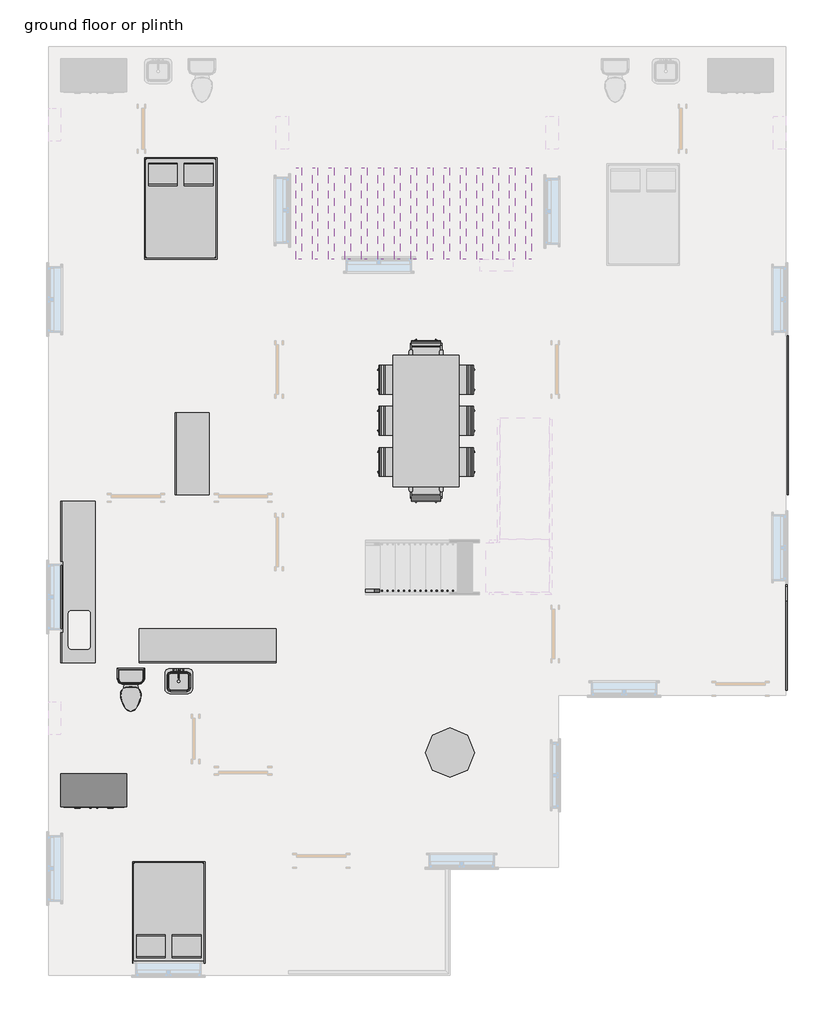
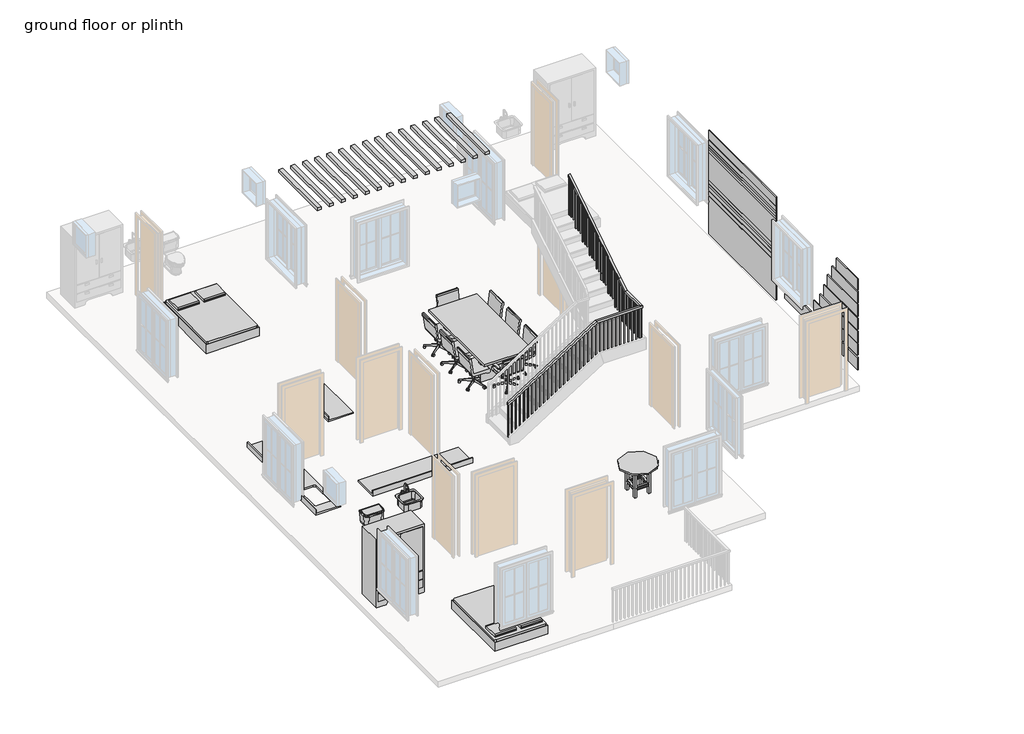
# One storey, part 2 of 3: 33 furniture elements, 2 flow terminals, 1 railing.
"""IFC4 building model written with IfcOpenShell, lengths in millimetres."""

from ifc_helpers import new_model, si_unit, frame, origin, place, context, project, spatial, polyline, outline, extrude, faceted_brep, transform, mapped, element, save
from components import flow_terminal_8d9ea526, toilet_domestic_3d_toilet_domestic_3d_ba6479b0, toilet_domestic_3d_toilet_domestic_3d_30431060, furniture_b58f7881, casework_1_casework_1_f574b021, casework_10_casework_1_3750556f, casework_11_casework_1_2f257332, casework_12_casework_1_dcbad799, casework_13_casework_1_b548bcc5, casework_14_casework_1_ad7f4f76, casework_16_casework_16_0ac3b185, casework_17_casework_17_3fc012a0, casework_18_casework_1_4256c183, casework_2_casework_1_1fe19027, casework_3_casework_1_f196c302, casework_4_casework_1_a5b175c9, casework_5_casework_1_a4356d40, casework_6_casework_1_aba422e7, casework_7_casework_1_d1433357, casework_8_casework_1_82254010, casework_9_casework_1_7a666160, chair_task_chair_task_b7f3823b, chair_task_arms_chair_task_arms_fa5a08ef, furniture_c0b19bce, furniture_c0b61535, furniture_6f689152, furniture_ec754799, furniture_32cec9f0, furniture_82e269c4

model = new_model("IFC4")

# Units and contexts
model_context = context("Model", 3, world=origin())
ifc_project = project(units=[si_unit("LENGTHUNIT", "METRE", prefix="MILLI")], contexts=[model_context])

# Site, building, storey
site = spatial("IfcSite", under=ifc_project)
building = spatial("IfcBuilding", under=site)
storey = spatial("IfcBuildingStorey", under=building, Name="ground floor or plinth", Elevation=609.6)

# Flow terminals
placement = place(None, origin())
flow_terminal_shape = flow_terminal_8d9ea526(model_context)
element("IfcFlowTerminal", 1, ObjectType="Sink Vanity-Square : 20\" x 18\"", at=placement, inside=storey, context=model_context, shape_type="MappedRepresentation", body=[
    mapped(flow_terminal_shape, transform((3106.5030862, 5324.1042913, 609.6), x_axis=(1.0, 0.0, 0.0), y_axis=(0.0, 1.0, 0.0), z_axis=(0.0, 0.0, 1.0))),
])
toilet_domestic_3d_toilet_domestic_3d_shape = toilet_domestic_3d_toilet_domestic_3d_ba6479b0(model_context)
toilet_domestic_3d_toilet_domestic_3d_2_shape = toilet_domestic_3d_toilet_domestic_3d_30431060(model_context)
element("IfcFlowTerminal", 2, ObjectType="Toilet-Domestic-3D : Toilet-Domestic-3D", at=placement, inside=storey, context=model_context, shape_type="MappedRepresentation", body=[
    mapped(toilet_domestic_3d_toilet_domestic_3d_shape, transform((2233.1923267, 5021.6496924, 609.6), x_axis=(1.0, 0.0, 0.0), y_axis=(0.0, 1.0, 0.0), z_axis=(0.0, 0.0, 1.0))),
    mapped(toilet_domestic_3d_toilet_domestic_3d_2_shape, transform((2233.1923267, 5021.6496924, 609.6), x_axis=(1.0, 0.0, 0.0), y_axis=(0.0, 1.0, 0.0), z_axis=(0.0, 0.0, 1.0))),
])

# Furniture
furniture_shape = furniture_b58f7881(model_context)
element("IfcFurniture", 3, ObjectType="Bed-Box : Double 53\" x 74\"", at=placement, inside=storey, context=model_context, shape_type="MappedRepresentation", body=[
    mapped(furniture_shape, transform((2821.1398677, 14273.0792006, 609.6), x_axis=(1.0, 0.0, 0.0), y_axis=(0.0, 1.0, 0.0), z_axis=(0.0, 0.0, 1.0))),
])
element("IfcFurniture", 4, ObjectType="Bed-Box : Double 53\" x 74\"", at=placement, inside=storey, context=model_context, shape_type="MappedRepresentation", body=[
    mapped(furniture_shape, transform((3277.1947857, 761.3201842, 609.6), x_axis=(-1.0, 0.0, 0.0), y_axis=(0.0, -1.0, 0.0), z_axis=(0.0, 0.0, 1.0))),
])
casework_1_casework_1_shape = casework_1_casework_1_f574b021(model_context)
element("IfcFurniture", 5, ObjectType="Casework 1 : Casework 1", at=placement, inside=storey, context=model_context, shape_type="MappedRepresentation", body=[
    mapped(casework_1_casework_1_shape, transform((0.0, 0.0, 0.0), x_axis=(1.0, 0.0, 0.0), y_axis=(0.0, 1.0, 0.0), z_axis=(0.0, 0.0, 1.0))),
])
casework_10_casework_1_shape = casework_10_casework_1_3750556f(model_context)
element("IfcFurniture", 6, ObjectType="Casework 10 : Casework 1", at=placement, inside=storey, context=model_context, shape_type="MappedRepresentation", body=[
    mapped(casework_10_casework_1_shape, transform((0.0, 0.0, 0.0), x_axis=(1.0, 0.0, 0.0), y_axis=(0.0, 1.0, 0.0), z_axis=(0.0, 0.0, 1.0))),
])
casework_11_casework_1_shape = casework_11_casework_1_2f257332(model_context)
element("IfcFurniture", 7, ObjectType="Casework 11 : Casework 1", at=placement, inside=storey, context=model_context, shape_type="MappedRepresentation", body=[
    mapped(casework_11_casework_1_shape, transform((0.0, 0.0, 0.0), x_axis=(1.0, 0.0, 0.0), y_axis=(0.0, 1.0, 0.0), z_axis=(0.0, 0.0, 1.0))),
])
casework_12_casework_1_shape = casework_12_casework_1_dcbad799(model_context)
element("IfcFurniture", 8, ObjectType="Casework 12 : Casework 1", at=placement, inside=storey, context=model_context, shape_type="MappedRepresentation", body=[
    mapped(casework_12_casework_1_shape, transform((0.0, 0.0, 0.0), x_axis=(1.0, 0.0, 0.0), y_axis=(0.0, 1.0, 0.0), z_axis=(0.0, 0.0, 1.0))),
])
casework_13_casework_1_shape = casework_13_casework_1_b548bcc5(model_context)
element("IfcFurniture", 9, ObjectType="Casework 13 : Casework 1", at=placement, inside=storey, context=model_context, shape_type="MappedRepresentation", body=[
    mapped(casework_13_casework_1_shape, transform((0.0, 0.0, 0.0), x_axis=(1.0, 0.0, 0.0), y_axis=(0.0, 1.0, 0.0), z_axis=(0.0, 0.0, 1.0))),
])
casework_14_casework_1_shape = casework_14_casework_1_ad7f4f76(model_context)
element("IfcFurniture", 10, ObjectType="Casework 14 : Casework 1", at=placement, inside=storey, context=model_context, shape_type="MappedRepresentation", body=[
    mapped(casework_14_casework_1_shape, transform((0.0, 0.0, 0.0), x_axis=(1.0, 0.0, 0.0), y_axis=(0.0, 1.0, 0.0), z_axis=(0.0, 0.0, 1.0))),
])
casework_16_casework_16_shape = casework_16_casework_16_0ac3b185(model_context)
element("IfcFurniture", 11, ObjectType="Casework 16 : Casework 16", at=placement, inside=storey, context=model_context, shape_type="MappedRepresentation", body=[
    mapped(casework_16_casework_16_shape, transform((0.0, 0.0, 0.0), x_axis=(1.0, 0.0, 0.0), y_axis=(0.0, 1.0, 0.0), z_axis=(0.0, 0.0, 1.0))),
])
casework_17_casework_17_shape = casework_17_casework_17_3fc012a0(model_context)
element("IfcFurniture", 12, ObjectType="Casework 17 : Casework 17", at=placement, inside=storey, context=model_context, shape_type="MappedRepresentation", body=[
    mapped(casework_17_casework_17_shape, transform((0.0, 0.0, 0.0), x_axis=(1.0, 0.0, 0.0), y_axis=(0.0, 1.0, 0.0), z_axis=(0.0, 0.0, 1.0))),
])
casework_18_casework_1_shape = casework_18_casework_1_4256c183(model_context)
element("IfcFurniture", 13, ObjectType="Casework 18 : Casework 1", at=placement, inside=storey, context=model_context, shape_type="MappedRepresentation", body=[
    mapped(casework_18_casework_1_shape, transform((0.0, 0.0, 0.0), x_axis=(1.0, 0.0, 0.0), y_axis=(0.0, 1.0, 0.0), z_axis=(0.0, 0.0, 1.0))),
])
casework_2_casework_1_shape = casework_2_casework_1_1fe19027(model_context)
element("IfcFurniture", 14, ObjectType="Casework 2 : Casework 1", at=placement, inside=storey, context=model_context, shape_type="MappedRepresentation", body=[
    mapped(casework_2_casework_1_shape, transform((0.0, 0.0, 0.0), x_axis=(1.0, 0.0, 0.0), y_axis=(0.0, 1.0, 0.0), z_axis=(0.0, 0.0, 1.0))),
])
casework_3_casework_1_shape = casework_3_casework_1_f196c302(model_context)
element("IfcFurniture", 15, ObjectType="Casework 3 : Casework 1", at=placement, inside=storey, context=model_context, shape_type="MappedRepresentation", body=[
    mapped(casework_3_casework_1_shape, transform((0.0, 0.0, 0.0), x_axis=(1.0, 0.0, 0.0), y_axis=(0.0, 1.0, 0.0), z_axis=(0.0, 0.0, 1.0))),
])
casework_4_casework_1_shape = casework_4_casework_1_a5b175c9(model_context)
element("IfcFurniture", 16, ObjectType="Casework 4 : Casework 1", at=placement, inside=storey, context=model_context, shape_type="MappedRepresentation", body=[
    mapped(casework_4_casework_1_shape, transform((0.0, 0.0, 0.0), x_axis=(1.0, 0.0, 0.0), y_axis=(0.0, 1.0, 0.0), z_axis=(0.0, 0.0, 1.0))),
])
casework_5_casework_1_shape = casework_5_casework_1_a4356d40(model_context)
element("IfcFurniture", 17, ObjectType="Casework 5 : Casework 1", at=placement, inside=storey, context=model_context, shape_type="MappedRepresentation", body=[
    mapped(casework_5_casework_1_shape, transform((0.0, 0.0, 0.0), x_axis=(1.0, 0.0, 0.0), y_axis=(0.0, 1.0, 0.0), z_axis=(0.0, 0.0, 1.0))),
])
casework_6_casework_1_shape = casework_6_casework_1_aba422e7(model_context)
element("IfcFurniture", 18, ObjectType="Casework 6 : Casework 1", at=placement, inside=storey, context=model_context, shape_type="MappedRepresentation", body=[
    mapped(casework_6_casework_1_shape, transform((0.0, 0.0, 0.0), x_axis=(1.0, 0.0, 0.0), y_axis=(0.0, 1.0, 0.0), z_axis=(0.0, 0.0, 1.0))),
])
casework_7_casework_1_shape = casework_7_casework_1_d1433357(model_context)
element("IfcFurniture", 19, ObjectType="Casework 7 : Casework 1", at=placement, inside=storey, context=model_context, shape_type="MappedRepresentation", body=[
    mapped(casework_7_casework_1_shape, transform((0.0, 0.0, 0.0), x_axis=(1.0, 0.0, 0.0), y_axis=(0.0, 1.0, 0.0), z_axis=(0.0, 0.0, 1.0))),
])
casework_8_casework_1_shape = casework_8_casework_1_82254010(model_context)
element("IfcFurniture", 20, ObjectType="Casework 8 : Casework 1", at=placement, inside=storey, context=model_context, shape_type="MappedRepresentation", body=[
    mapped(casework_8_casework_1_shape, transform((0.0, 0.0, 0.0), x_axis=(1.0, 0.0, 0.0), y_axis=(0.0, 1.0, 0.0), z_axis=(0.0, 0.0, 1.0))),
])
casework_9_casework_1_shape = casework_9_casework_1_7a666160(model_context)
element("IfcFurniture", 21, ObjectType="Casework 9 : Casework 1", at=placement, inside=storey, context=model_context, shape_type="MappedRepresentation", body=[
    mapped(casework_9_casework_1_shape, transform((0.0, 0.0, 0.0), x_axis=(1.0, 0.0, 0.0), y_axis=(0.0, 1.0, 0.0), z_axis=(0.0, 0.0, 1.0))),
])
chair_task_chair_task_shape = chair_task_chair_task_b7f3823b(model_context)
element("IfcFurniture", 22, ObjectType="Chair-Task : Chair-Task", at=placement, inside=storey, context=model_context, shape_type="MappedRepresentation", body=[
    mapped(chair_task_chair_task_shape, transform((7078.3464251, 10242.6405121, 609.6), x_axis=(0.0, -1.0, 0.0), y_axis=(1.0, 0.0, 0.0), z_axis=(0.0, 0.0, 1.0))),
])
element("IfcFurniture", 23, ObjectType="Chair-Task : Chair-Task", at=placement, inside=storey, context=model_context, shape_type="MappedRepresentation", body=[
    mapped(chair_task_chair_task_shape, transform((7078.3464251, 11004.6405121, 609.6), x_axis=(0.0, -1.0, 0.0), y_axis=(1.0, 0.0, 0.0), z_axis=(0.0, 0.0, 1.0))),
])
element("IfcFurniture", 24, ObjectType="Chair-Task : Chair-Task", at=placement, inside=storey, context=model_context, shape_type="MappedRepresentation", body=[
    mapped(chair_task_chair_task_shape, transform((8335.4382284, 9960.6588728, 609.6), x_axis=(0.0, 1.0, 0.0), y_axis=(-1.0, 0.0, 0.0), z_axis=(0.0, 0.0, 1.0))),
])
element("IfcFurniture", 25, ObjectType="Chair-Task : Chair-Task", at=placement, inside=storey, context=model_context, shape_type="MappedRepresentation", body=[
    mapped(chair_task_chair_task_shape, transform((8335.4382284, 10722.6588728, 609.6), x_axis=(0.0, 1.0, 0.0), y_axis=(-1.0, 0.0, 0.0), z_axis=(0.0, 0.0, 1.0))),
])
element("IfcFurniture", 26, ObjectType="Chair-Task : Chair-Task", at=placement, inside=storey, context=model_context, shape_type="MappedRepresentation", body=[
    mapped(chair_task_chair_task_shape, transform((7078.3464251, 9480.6405121, 609.6), x_axis=(0.0, -1.0, 0.0), y_axis=(1.0, 0.0, 0.0), z_axis=(0.0, 0.0, 1.0))),
])
element("IfcFurniture", 27, ObjectType="Chair-Task : Chair-Task", at=placement, inside=storey, context=model_context, shape_type="MappedRepresentation", body=[
    mapped(chair_task_chair_task_shape, transform((8335.4382284, 9198.6588728, 609.6), x_axis=(0.0, 1.0, 0.0), y_axis=(-1.0, 0.0, 0.0), z_axis=(0.0, 0.0, 1.0))),
])
chair_task_arms_chair_task_arms_shape = chair_task_arms_chair_task_arms_fa5a08ef(model_context)
element("IfcFurniture", 28, ObjectType="Chair-Task Arms : Chair-Task Arms", at=placement, inside=storey, context=model_context, shape_type="MappedRepresentation", body=[
    mapped(chair_task_arms_chair_task_arms_shape, transform((7565.9015071, 8863.5037908, 609.6), x_axis=(1.0, 0.0, 0.0), y_axis=(0.0, 1.0, 0.0), z_axis=(0.0, 0.0, 1.0))),
])
element("IfcFurniture", 29, ObjectType="Chair-Task Arms : Chair-Task Arms", at=placement, inside=storey, context=model_context, shape_type="MappedRepresentation", body=[
    mapped(chair_task_arms_chair_task_arms_shape, transform((7847.8831464, 11339.7955941, 609.6), x_axis=(-1.0, 0.0, 0.0), y_axis=(0.0, -1.0, 0.0), z_axis=(0.0, 0.0, 1.0))),
])
furniture_2_shape = furniture_c0b19bce(model_context)
element("IfcFurniture", 30, ObjectType="Counter Top : 24\" Depth", at=placement, inside=storey, context=model_context, shape_type="MappedRepresentation", body=[
    mapped(furniture_2_shape, transform((3725.1300316, 5618.5496924, 609.6), x_axis=(-1.0, 0.0, 0.0), y_axis=(0.0, -1.0, 0.0), z_axis=(0.0, 0.0, 1.0))),
])
furniture_3_shape = furniture_c0b61535(model_context)
element("IfcFurniture", 31, ObjectType="Counter Top w Sink Hole : 24\" Depth", at=placement, inside=storey, context=model_context, shape_type="MappedRepresentation", body=[
    mapped(furniture_3_shape, transform((937.7923267, 6819.0119875, 609.6), x_axis=(0.0, 1.0, 0.0), y_axis=(-1.0, 0.0, 0.0), z_axis=(0.0, 0.0, 1.0))),
])
furniture_4_shape = furniture_6f689152(model_context)
element("IfcFurniture", 32, ObjectType="Table-Conference2 w Chairs : 48\" x 144\"", at=placement, inside=storey, context=model_context, shape_type="MappedRepresentation", body=[
    mapped(furniture_4_shape, transform((7706.8923267, 10101.6496924, 609.6), x_axis=(0.0, 1.0, 0.0), y_axis=(-1.0, 0.0, 0.0), z_axis=(0.0, 0.0, 1.0))),
])
furniture_5_shape = furniture_ec754799(model_context)
element("IfcFurniture", 33, ObjectType="Table-Dining Round : 36\" Diameter", at=placement, inside=storey, context=model_context, shape_type="MappedRepresentation", body=[
    mapped(furniture_5_shape, transform((8047.7103595, 4139.728381, 609.6), x_axis=(1.0, 0.0, 0.0), y_axis=(0.0, 1.0, 0.0), z_axis=(0.0, 0.0, 1.0))),
])
furniture_6_shape = furniture_32cec9f0(model_context)
element("IfcFurniture", 34, ObjectType="Vanity Counter Top : 24\" Depth", at=placement, inside=storey, context=model_context, shape_type="MappedRepresentation", body=[
    mapped(furniture_6_shape, transform((3052.3423267, 9930.5119875, 609.6), x_axis=(0.0, 1.0, 0.0), y_axis=(-1.0, 0.0, 0.0), z_axis=(0.0, 0.0, 1.0))),
])
furniture_7_shape = furniture_82e269c4(model_context)
element("IfcFurniture", 35, ObjectType="Wardrobe : 48\" x 72\" x 24\"", at=placement, inside=storey, context=model_context, shape_type="MappedRepresentation", body=[
    mapped(furniture_7_shape, transform((1816.5855866, 3840.088502, 609.6), x_axis=(1.0, 0.0, 0.0), y_axis=(0.0, 1.0, 0.0), z_axis=(0.0, 0.0, 1.0))),
])

# Railing
element("IfcRailing", 36, ObjectType="Handrail - Rectangular", at=placement, inside=storey, context=model_context, shape_type="SolidModel", body=[
    faceted_brep([(6584.2175025, 6979.4147181, 1701.8), (6584.2175025, 6979.4147181, 1641.586276), (6584.2175025, 6928.6147181, 1641.586276), (6584.2175025, 6928.6147181, 1701.8), (8819.4175025, 6979.4147181, 3124.2), (8834.2104975, 6979.4147181, 3073.4), (8834.2104975, 6928.6147181, 3073.4), (8819.4175025, 6928.6147181, 3124.2), (9942.0923267, 6979.4147181, 3124.2), (9942.0923267, 6979.4147181, 3073.4), (9992.8923267, 6928.6147181, 3073.4), (9992.8923267, 6928.6147181, 3124.2), (9942.0923267, 7614.4147181, 3124.2), (9942.0923267, 7629.207713, 3073.4), (9992.8923267, 7629.207713, 3073.4), (9992.8923267, 7614.4147181, 3124.2), (9942.0923267, 7893.8147181, 3302.0), (9942.0923267, 7921.0879931, 3259.1419964), (9992.8923267, 7921.0879931, 3259.1419964), (9992.8923267, 7893.8147181, 3302.0), (9942.0923267, 10129.0147181, 4724.4), (9992.8923267, 10129.0147181, 4724.4), (9992.8923267, 10129.0147181, 4664.186276), (9942.0923267, 10129.0147181, 4664.186276)], [[[0, 1, 2, 3]], [[1, 0, 4, 5]], [[2, 1, 5, 6]], [[3, 2, 6, 7]], [[0, 3, 7, 4]], [[5, 4, 8, 9]], [[6, 5, 9, 10]], [[7, 6, 10, 11]], [[4, 7, 11, 8]], [[9, 8, 12, 13]], [[10, 9, 13, 14]], [[11, 10, 14, 15]], [[8, 11, 15, 12]], [[13, 12, 16, 17]], [[14, 13, 17, 18]], [[15, 14, 18, 19]], [[12, 15, 19, 16]], [[20, 21, 22, 23]], [[17, 16, 20, 23]], [[18, 17, 23, 22]], [[19, 18, 22, 21]], [[16, 19, 21, 20]]]),
    extrude(outline(polyline([(10017.8897181, 4593.4703669), (10036.9397181, 4605.5930941), (10036.9397181, 3632.2), (10017.8897181, 3632.2), (10017.8897181, 4593.4703669)])), frame((9957.9673267, 0.0, 0.0), z_axis=(1.0, 0.0, 0.0), x_axis=(0.0, 1.0, 0.0)), (0.0, 0.0, 1.0), 19.05),
    extrude(outline(polyline([(9916.2897181, 4528.8158214), (9935.3397181, 4540.9385487), (9935.3397181, 3632.2), (9916.2897181, 3632.2), (9916.2897181, 4528.8158214)])), frame((9957.9673267, 0.0, 0.0), z_axis=(1.0, 0.0, 0.0), x_axis=(0.0, 1.0, 0.0)), (0.0, 0.0, 1.0), 19.05),
    extrude(outline(polyline([(9814.6897181, 4464.161276), (9833.7397181, 4476.2840032), (9833.7397181, 3454.4), (9814.6897181, 3454.4), (9814.6897181, 4464.161276)])), frame((9957.9673267, 0.0, 0.0), z_axis=(1.0, 0.0, 0.0), x_axis=(0.0, 1.0, 0.0)), (0.0, 0.0, 1.0), 19.05),
    extrude(outline(polyline([(9713.0897181, 4399.5067305), (9732.1397181, 4411.6294578), (9732.1397181, 3454.4), (9713.0897181, 3454.4), (9713.0897181, 4399.5067305)])), frame((9957.9673267, 0.0, 0.0), z_axis=(1.0, 0.0, 0.0), x_axis=(0.0, 1.0, 0.0)), (0.0, 0.0, 1.0), 19.05),
    extrude(outline(polyline([(9611.4897181, 4334.8521851), (9630.5397181, 4346.9749123), (9630.5397181, 3454.4), (9611.4897181, 3454.4), (9611.4897181, 4334.8521851)])), frame((9957.9673267, 0.0, 0.0), z_axis=(1.0, 0.0, 0.0), x_axis=(0.0, 1.0, 0.0)), (0.0, 0.0, 1.0), 19.05),
    extrude(outline(polyline([(9509.8897181, 4270.1976396), (9528.9397181, 4282.3203669), (9528.9397181, 3276.6), (9509.8897181, 3276.6), (9509.8897181, 4270.1976396)])), frame((9957.9673267, 0.0, 0.0), z_axis=(1.0, 0.0, 0.0), x_axis=(0.0, 1.0, 0.0)), (0.0, 0.0, 1.0), 19.05),
    extrude(outline(polyline([(9408.2897181, 4205.5430941), (9427.3397181, 4217.6658214), (9427.3397181, 3276.6), (9408.2897181, 3276.6), (9408.2897181, 4205.5430941)])), frame((9957.9673267, 0.0, 0.0), z_axis=(1.0, 0.0, 0.0), x_axis=(0.0, 1.0, 0.0)), (0.0, 0.0, 1.0), 19.05),
    extrude(outline(polyline([(9306.6897181, 4140.8885487), (9325.7397181, 4153.011276), (9325.7397181, 3276.6), (9306.6897181, 3276.6), (9306.6897181, 4140.8885487)])), frame((9957.9673267, 0.0, 0.0), z_axis=(1.0, 0.0, 0.0), x_axis=(0.0, 1.0, 0.0)), (0.0, 0.0, 1.0), 19.05),
    extrude(outline(polyline([(9205.0897181, 4076.2340032), (9224.1397181, 4088.3567305), (9224.1397181, 3098.8), (9205.0897181, 3098.8), (9205.0897181, 4076.2340032)])), frame((9957.9673267, 0.0, 0.0), z_axis=(1.0, 0.0, 0.0), x_axis=(0.0, 1.0, 0.0)), (0.0, 0.0, 1.0), 19.05),
    extrude(outline(polyline([(9103.4897181, 4011.5794578), (9122.5397181, 4023.7021851), (9122.5397181, 3098.8), (9103.4897181, 3098.8), (9103.4897181, 4011.5794578)])), frame((9957.9673267, 0.0, 0.0), z_axis=(1.0, 0.0, 0.0), x_axis=(0.0, 1.0, 0.0)), (0.0, 0.0, 1.0), 19.05),
    extrude(outline(polyline([(9001.8897181, 3946.9249123), (9020.9397181, 3959.0476396), (9020.9397181, 3098.8), (9001.8897181, 3098.8), (9001.8897181, 3946.9249123)])), frame((9957.9673267, 0.0, 0.0), z_axis=(1.0, 0.0, 0.0), x_axis=(0.0, 1.0, 0.0)), (0.0, 0.0, 1.0), 19.05),
    extrude(outline(polyline([(8900.2897181, 3882.2703669), (8919.3397181, 3894.3930941), (8919.3397181, 2921.0), (8900.2897181, 2921.0), (8900.2897181, 3882.2703669)])), frame((9957.9673267, 0.0, 0.0), z_axis=(1.0, 0.0, 0.0), x_axis=(0.0, 1.0, 0.0)), (0.0, 0.0, 1.0), 19.05),
    extrude(outline(polyline([(8798.6897181, 3817.6158214), (8817.7397181, 3829.7385487), (8817.7397181, 2921.0), (8798.6897181, 2921.0), (8798.6897181, 3817.6158214)])), frame((9957.9673267, 0.0, 0.0), z_axis=(1.0, 0.0, 0.0), x_axis=(0.0, 1.0, 0.0)), (0.0, 0.0, 1.0), 19.05),
    extrude(outline(polyline([(8697.0897181, 3752.961276), (8716.1397181, 3765.0840032), (8716.1397181, 2743.2), (8697.0897181, 2743.2), (8697.0897181, 3752.961276)])), frame((9957.9673267, 0.0, 0.0), z_axis=(1.0, 0.0, 0.0), x_axis=(0.0, 1.0, 0.0)), (0.0, 0.0, 1.0), 19.05),
    extrude(outline(polyline([(8595.4897181, 3688.3067305), (8614.5397181, 3700.4294578), (8614.5397181, 2743.2), (8595.4897181, 2743.2), (8595.4897181, 3688.3067305)])), frame((9957.9673267, 0.0, 0.0), z_axis=(1.0, 0.0, 0.0), x_axis=(0.0, 1.0, 0.0)), (0.0, 0.0, 1.0), 19.05),
    extrude(outline(polyline([(8493.8897181, 3623.6521851), (8512.9397181, 3635.7749123), (8512.9397181, 2743.2), (8493.8897181, 2743.2), (8493.8897181, 3623.6521851)])), frame((9957.9673267, 0.0, 0.0), z_axis=(1.0, 0.0, 0.0), x_axis=(0.0, 1.0, 0.0)), (0.0, 0.0, 1.0), 19.05),
    extrude(outline(polyline([(8392.2897181, 3558.9976396), (8411.3397181, 3571.1203669), (8411.3397181, 2565.4), (8392.2897181, 2565.4), (8392.2897181, 3558.9976396)])), frame((9957.9673267, 0.0, 0.0), z_axis=(1.0, 0.0, 0.0), x_axis=(0.0, 1.0, 0.0)), (0.0, 0.0, 1.0), 19.05),
    extrude(outline(polyline([(8290.6897181, 3494.3430941), (8309.7397181, 3506.4658214), (8309.7397181, 2565.4), (8290.6897181, 2565.4), (8290.6897181, 3494.3430941)])), frame((9957.9673267, 0.0, 0.0), z_axis=(1.0, 0.0, 0.0), x_axis=(0.0, 1.0, 0.0)), (0.0, 0.0, 1.0), 19.05),
    extrude(outline(polyline([(8189.0897181, 3429.6885487), (8208.1397181, 3441.811276), (8208.1397181, 2565.4), (8189.0897181, 2565.4), (8189.0897181, 3429.6885487)])), frame((9957.9673267, 0.0, 0.0), z_axis=(1.0, 0.0, 0.0), x_axis=(0.0, 1.0, 0.0)), (0.0, 0.0, 1.0), 19.05),
    extrude(outline(polyline([(8087.4897181, 3365.0340032), (8106.5397181, 3377.1567305), (8106.5397181, 2387.6), (8087.4897181, 2387.6), (8087.4897181, 3365.0340032)])), frame((9957.9673267, 0.0, 0.0), z_axis=(1.0, 0.0, 0.0), x_axis=(0.0, 1.0, 0.0)), (0.0, 0.0, 1.0), 19.05),
    extrude(outline(polyline([(7985.8897181, 3300.3794578), (8004.9397181, 3312.5021851), (8004.9397181, 2387.6), (7985.8897181, 2387.6), (7985.8897181, 3300.3794578)])), frame((9957.9673267, 0.0, 0.0), z_axis=(1.0, 0.0, 0.0), x_axis=(0.0, 1.0, 0.0)), (0.0, 0.0, 1.0), 19.05),
    extrude(outline(polyline([(7858.8897181, 3219.561276), (7877.9397181, 3231.6840032), (7877.9397181, 2209.8), (7858.8897181, 2209.8), (7858.8897181, 3219.561276)])), frame((9957.9673267, 0.0, 0.0), z_axis=(1.0, 0.0, 0.0), x_axis=(0.0, 1.0, 0.0)), (0.0, 0.0, 1.0), 19.05),
    extrude(outline(polyline([(7757.2897181, 3154.9067305), (7776.3397181, 3167.0294578), (7776.3397181, 2209.8), (7757.2897181, 2209.8), (7757.2897181, 3154.9067305)])), frame((9957.9673267, 0.0, 0.0), z_axis=(1.0, 0.0, 0.0), x_axis=(0.0, 1.0, 0.0)), (0.0, 0.0, 1.0), 19.05),
    extrude(outline(polyline([(7655.6897181, 3090.2521851), (7674.7397181, 3102.3749123), (7674.7397181, 2209.8), (7655.6897181, 2209.8), (7655.6897181, 3090.2521851)])), frame((9957.9673267, 0.0, 0.0), z_axis=(1.0, 0.0, 0.0), x_axis=(0.0, 1.0, 0.0)), (0.0, 0.0, 1.0), 19.05),
    extrude(outline(polyline([(9977.0173267, 7554.0897181), (9957.9673267, 7554.0897181), (9957.9673267, 7573.1397181), (9977.0173267, 7573.1397181), (9977.0173267, 7554.0897181)])), frame((0.0, 0.0, 2209.8), z_axis=(0.0, 0.0, 1.0), x_axis=(1.0, 0.0, 0.0)), (0.0, 0.0, 1.0), 863.6),
    extrude(outline(polyline([(9977.0173267, 7452.4897181), (9957.9673267, 7452.4897181), (9957.9673267, 7471.5397181), (9977.0173267, 7471.5397181), (9977.0173267, 7452.4897181)])), frame((0.0, 0.0, 2209.8), z_axis=(0.0, 0.0, 1.0), x_axis=(1.0, 0.0, 0.0)), (0.0, 0.0, 1.0), 863.6),
    extrude(outline(polyline([(9977.0173267, 7350.8897181), (9957.9673267, 7350.8897181), (9957.9673267, 7369.9397181), (9977.0173267, 7369.9397181), (9977.0173267, 7350.8897181)])), frame((0.0, 0.0, 2209.8), z_axis=(0.0, 0.0, 1.0), x_axis=(1.0, 0.0, 0.0)), (0.0, 0.0, 1.0), 863.6),
    extrude(outline(polyline([(9977.0173267, 7249.2897181), (9957.9673267, 7249.2897181), (9957.9673267, 7268.3397181), (9977.0173267, 7268.3397181), (9977.0173267, 7249.2897181)])), frame((0.0, 0.0, 2209.8), z_axis=(0.0, 0.0, 1.0), x_axis=(1.0, 0.0, 0.0)), (0.0, 0.0, 1.0), 863.6),
    extrude(outline(polyline([(9977.0173267, 7147.6897181), (9957.9673267, 7147.6897181), (9957.9673267, 7166.7397181), (9977.0173267, 7166.7397181), (9977.0173267, 7147.6897181)])), frame((0.0, 0.0, 2209.8), z_axis=(0.0, 0.0, 1.0), x_axis=(1.0, 0.0, 0.0)), (0.0, 0.0, 1.0), 863.6),
    extrude(outline(polyline([(9977.0173267, 7046.0897181), (9957.9673267, 7046.0897181), (9957.9673267, 7065.1397181), (9977.0173267, 7065.1397181), (9977.0173267, 7046.0897181)])), frame((0.0, 0.0, 2209.8), z_axis=(0.0, 0.0, 1.0), x_axis=(1.0, 0.0, 0.0)), (0.0, 0.0, 1.0), 863.6),
    extrude(outline(polyline([(9927.4925025, 6944.4897181), (9927.4925025, 6963.5397181), (9946.5425025, 6963.5397181), (9946.5425025, 6944.4897181), (9927.4925025, 6944.4897181)])), frame((0.0, 0.0, 2209.8), z_axis=(0.0, 0.0, 1.0), x_axis=(1.0, 0.0, 0.0)), (0.0, 0.0, 1.0), 863.6),
    extrude(outline(polyline([(9825.8925025, 6944.4897181), (9825.8925025, 6963.5397181), (9844.9425025, 6963.5397181), (9844.9425025, 6944.4897181), (9825.8925025, 6944.4897181)])), frame((0.0, 0.0, 2209.8), z_axis=(0.0, 0.0, 1.0), x_axis=(1.0, 0.0, 0.0)), (0.0, 0.0, 1.0), 863.6),
    extrude(outline(polyline([(9724.2925025, 6944.4897181), (9724.2925025, 6963.5397181), (9743.3425025, 6963.5397181), (9743.3425025, 6944.4897181), (9724.2925025, 6944.4897181)])), frame((0.0, 0.0, 2209.8), z_axis=(0.0, 0.0, 1.0), x_axis=(1.0, 0.0, 0.0)), (0.0, 0.0, 1.0), 863.6),
    extrude(outline(polyline([(9622.6925025, 6944.4897181), (9622.6925025, 6963.5397181), (9641.7425025, 6963.5397181), (9641.7425025, 6944.4897181), (9622.6925025, 6944.4897181)])), frame((0.0, 0.0, 2209.8), z_axis=(0.0, 0.0, 1.0), x_axis=(1.0, 0.0, 0.0)), (0.0, 0.0, 1.0), 863.6),
    extrude(outline(polyline([(9521.0925025, 6944.4897181), (9521.0925025, 6963.5397181), (9540.1425025, 6963.5397181), (9540.1425025, 6944.4897181), (9521.0925025, 6944.4897181)])), frame((0.0, 0.0, 2209.8), z_axis=(0.0, 0.0, 1.0), x_axis=(1.0, 0.0, 0.0)), (0.0, 0.0, 1.0), 863.6),
    extrude(outline(polyline([(9419.4925025, 6944.4897181), (9419.4925025, 6963.5397181), (9438.5425025, 6963.5397181), (9438.5425025, 6944.4897181), (9419.4925025, 6944.4897181)])), frame((0.0, 0.0, 2209.8), z_axis=(0.0, 0.0, 1.0), x_axis=(1.0, 0.0, 0.0)), (0.0, 0.0, 1.0), 863.6),
    extrude(outline(polyline([(9317.8925025, 6944.4897181), (9317.8925025, 6963.5397181), (9336.9425025, 6963.5397181), (9336.9425025, 6944.4897181), (9317.8925025, 6944.4897181)])), frame((0.0, 0.0, 2209.8), z_axis=(0.0, 0.0, 1.0), x_axis=(1.0, 0.0, 0.0)), (0.0, 0.0, 1.0), 863.6),
    extrude(outline(polyline([(9216.2925025, 6944.4897181), (9216.2925025, 6963.5397181), (9235.3425025, 6963.5397181), (9235.3425025, 6944.4897181), (9216.2925025, 6944.4897181)])), frame((0.0, 0.0, 2209.8), z_axis=(0.0, 0.0, 1.0), x_axis=(1.0, 0.0, 0.0)), (0.0, 0.0, 1.0), 863.6),
    extrude(outline(polyline([(9114.6925025, 6944.4897181), (9114.6925025, 6963.5397181), (9133.7425025, 6963.5397181), (9133.7425025, 6944.4897181), (9114.6925025, 6944.4897181)])), frame((0.0, 0.0, 2209.8), z_axis=(0.0, 0.0, 1.0), x_axis=(1.0, 0.0, 0.0)), (0.0, 0.0, 1.0), 863.6),
    extrude(outline(polyline([(9013.0925025, 6944.4897181), (9013.0925025, 6963.5397181), (9032.1425025, 6963.5397181), (9032.1425025, 6944.4897181), (9013.0925025, 6944.4897181)])), frame((0.0, 0.0, 2209.8), z_axis=(0.0, 0.0, 1.0), x_axis=(1.0, 0.0, 0.0)), (0.0, 0.0, 1.0), 863.6),
    extrude(outline(polyline([(8911.4925025, 6944.4897181), (8911.4925025, 6963.5397181), (8930.5425025, 6963.5397181), (8930.5425025, 6944.4897181), (8911.4925025, 6944.4897181)])), frame((0.0, 0.0, 2209.8), z_axis=(0.0, 0.0, 1.0), x_axis=(1.0, 0.0, 0.0)), (0.0, 0.0, 1.0), 863.6),
    extrude(outline(polyline([(3005.3930941, 8727.3425025), (2993.2703669, 8708.2925025), (2032.0, 8708.2925025), (2032.0, 8727.3425025), (3005.3930941, 8727.3425025)])), frame((0.0, 6944.4897181, 0.0), z_axis=(0.0, 1.0, 0.0), x_axis=(0.0, 0.0, 1.0)), (0.0, 0.0, 1.0), 19.05),
    extrude(outline(polyline([(2940.7385487, 8625.7425025), (2928.6158214, 8606.6925025), (2032.0, 8606.6925025), (2032.0, 8625.7425025), (2940.7385487, 8625.7425025)])), frame((0.0, 6944.4897181, 0.0), z_axis=(0.0, 1.0, 0.0), x_axis=(0.0, 0.0, 1.0)), (0.0, 0.0, 1.0), 19.05),
    extrude(outline(polyline([(2876.0840032, 8524.1425025), (2863.961276, 8505.0925025), (1854.2, 8505.0925025), (1854.2, 8524.1425025), (2876.0840032, 8524.1425025)])), frame((0.0, 6944.4897181, 0.0), z_axis=(0.0, 1.0, 0.0), x_axis=(0.0, 0.0, 1.0)), (0.0, 0.0, 1.0), 19.05),
    extrude(outline(polyline([(2811.4294578, 8422.5425025), (2799.3067305, 8403.4925025), (1854.2, 8403.4925025), (1854.2, 8422.5425025), (2811.4294578, 8422.5425025)])), frame((0.0, 6944.4897181, 0.0), z_axis=(0.0, 1.0, 0.0), x_axis=(0.0, 0.0, 1.0)), (0.0, 0.0, 1.0), 19.05),
    extrude(outline(polyline([(2746.7749123, 8320.9425025), (2734.6521851, 8301.8925025), (1854.2, 8301.8925025), (1854.2, 8320.9425025), (2746.7749123, 8320.9425025)])), frame((0.0, 6944.4897181, 0.0), z_axis=(0.0, 1.0, 0.0), x_axis=(0.0, 0.0, 1.0)), (0.0, 0.0, 1.0), 19.05),
    extrude(outline(polyline([(2682.1203669, 8219.3425025), (2669.9976396, 8200.2925025), (1676.4, 8200.2925025), (1676.4, 8219.3425025), (2682.1203669, 8219.3425025)])), frame((0.0, 6944.4897181, 0.0), z_axis=(0.0, 1.0, 0.0), x_axis=(0.0, 0.0, 1.0)), (0.0, 0.0, 1.0), 19.05),
    extrude(outline(polyline([(2617.4658214, 8117.7425025), (2605.3430941, 8098.6925025), (1676.4, 8098.6925025), (1676.4, 8117.7425025), (2617.4658214, 8117.7425025)])), frame((0.0, 6944.4897181, 0.0), z_axis=(0.0, 1.0, 0.0), x_axis=(0.0, 0.0, 1.0)), (0.0, 0.0, 1.0), 19.05),
    extrude(outline(polyline([(2552.811276, 8016.1425025), (2540.6885487, 7997.0925025), (1676.4, 7997.0925025), (1676.4, 8016.1425025), (2552.811276, 8016.1425025)])), frame((0.0, 6944.4897181, 0.0), z_axis=(0.0, 1.0, 0.0), x_axis=(0.0, 0.0, 1.0)), (0.0, 0.0, 1.0), 19.05),
    extrude(outline(polyline([(2488.1567305, 7914.5425025), (2476.0340032, 7895.4925025), (1498.6, 7895.4925025), (1498.6, 7914.5425025), (2488.1567305, 7914.5425025)])), frame((0.0, 6944.4897181, 0.0), z_axis=(0.0, 1.0, 0.0), x_axis=(0.0, 0.0, 1.0)), (0.0, 0.0, 1.0), 19.05),
    extrude(outline(polyline([(2423.5021851, 7812.9425025), (2411.3794578, 7793.8925025), (1498.6, 7793.8925025), (1498.6, 7812.9425025), (2423.5021851, 7812.9425025)])), frame((0.0, 6944.4897181, 0.0), z_axis=(0.0, 1.0, 0.0), x_axis=(0.0, 0.0, 1.0)), (0.0, 0.0, 1.0), 19.05),
    extrude(outline(polyline([(2358.8476396, 7711.3425025), (2346.7249123, 7692.2925025), (1498.6, 7692.2925025), (1498.6, 7711.3425025), (2358.8476396, 7711.3425025)])), frame((0.0, 6944.4897181, 0.0), z_axis=(0.0, 1.0, 0.0), x_axis=(0.0, 0.0, 1.0)), (0.0, 0.0, 1.0), 19.05),
    extrude(outline(polyline([(2294.1930941, 7609.7425025), (2282.0703669, 7590.6925025), (1320.8, 7590.6925025), (1320.8, 7609.7425025), (2294.1930941, 7609.7425025)])), frame((0.0, 6944.4897181, 0.0), z_axis=(0.0, 1.0, 0.0), x_axis=(0.0, 0.0, 1.0)), (0.0, 0.0, 1.0), 19.05),
    extrude(outline(polyline([(2229.5385487, 7508.1425025), (2217.4158214, 7489.0925025), (1320.8, 7489.0925025), (1320.8, 7508.1425025), (2229.5385487, 7508.1425025)])), frame((0.0, 6944.4897181, 0.0), z_axis=(0.0, 1.0, 0.0), x_axis=(0.0, 0.0, 1.0)), (0.0, 0.0, 1.0), 19.05),
    extrude(outline(polyline([(2164.8840032, 7406.5425025), (2152.761276, 7387.4925025), (1143.0, 7387.4925025), (1143.0, 7406.5425025), (2164.8840032, 7406.5425025)])), frame((0.0, 6944.4897181, 0.0), z_axis=(0.0, 1.0, 0.0), x_axis=(0.0, 0.0, 1.0)), (0.0, 0.0, 1.0), 19.05),
    extrude(outline(polyline([(2100.2294578, 7304.9425025), (2088.1067305, 7285.8925025), (1143.0, 7285.8925025), (1143.0, 7304.9425025), (2100.2294578, 7304.9425025)])), frame((0.0, 6944.4897181, 0.0), z_axis=(0.0, 1.0, 0.0), x_axis=(0.0, 0.0, 1.0)), (0.0, 0.0, 1.0), 19.05),
    extrude(outline(polyline([(2035.5749123, 7203.3425025), (2023.4521851, 7184.2925025), (1143.0, 7184.2925025), (1143.0, 7203.3425025), (2035.5749123, 7203.3425025)])), frame((0.0, 6944.4897181, 0.0), z_axis=(0.0, 1.0, 0.0), x_axis=(0.0, 0.0, 1.0)), (0.0, 0.0, 1.0), 19.05),
    extrude(outline(polyline([(1970.9203669, 7101.7425025), (1958.7976396, 7082.6925025), (965.2, 7082.6925025), (965.2, 7101.7425025), (1970.9203669, 7101.7425025)])), frame((0.0, 6944.4897181, 0.0), z_axis=(0.0, 1.0, 0.0), x_axis=(0.0, 0.0, 1.0)), (0.0, 0.0, 1.0), 19.05),
    extrude(outline(polyline([(1906.2658214, 7000.1425025), (1894.1430941, 6981.0925025), (965.2, 6981.0925025), (965.2, 7000.1425025), (1906.2658214, 7000.1425025)])), frame((0.0, 6944.4897181, 0.0), z_axis=(0.0, 1.0, 0.0), x_axis=(0.0, 0.0, 1.0)), (0.0, 0.0, 1.0), 19.05),
    extrude(outline(polyline([(1841.611276, 6898.5425025), (1829.4885487, 6879.4925025), (965.2, 6879.4925025), (965.2, 6898.5425025), (1841.611276, 6898.5425025)])), frame((0.0, 6944.4897181, 0.0), z_axis=(0.0, 1.0, 0.0), x_axis=(0.0, 0.0, 1.0)), (0.0, 0.0, 1.0), 19.05),
    extrude(outline(polyline([(1776.9567305, 6796.9425025), (1764.8340032, 6777.8925025), (787.4, 6777.8925025), (787.4, 6796.9425025), (1776.9567305, 6796.9425025)])), frame((0.0, 6944.4897181, 0.0), z_axis=(0.0, 1.0, 0.0), x_axis=(0.0, 0.0, 1.0)), (0.0, 0.0, 1.0), 19.05),
    extrude(outline(polyline([(1712.3021851, 6695.3425025), (1700.1794578, 6676.2925025), (787.4, 6676.2925025), (787.4, 6695.3425025), (1712.3021851, 6695.3425025)])), frame((0.0, 6944.4897181, 0.0), z_axis=(0.0, 1.0, 0.0), x_axis=(0.0, 0.0, 1.0)), (0.0, 0.0, 1.0), 19.05),
    extrude(outline(polyline([(7884.2897181, 3235.7249123), (7903.3397181, 3247.8476396), (7903.3397181, 2209.8), (7884.2897181, 2209.8), (7884.2897181, 3235.7249123)])), frame((9957.9673267, 0.0, 0.0), z_axis=(1.0, 0.0, 0.0), x_axis=(0.0, 1.0, 0.0)), (0.0, 0.0, 1.0), 19.05),
    extrude(outline(polyline([(9957.9673267, 6944.4897181), (9957.9673267, 6963.5397181), (9977.0173267, 6963.5397181), (9977.0173267, 6944.4897181), (9957.9673267, 6944.4897181)])), frame((0.0, 0.0, 2209.8), z_axis=(0.0, 0.0, 1.0), x_axis=(1.0, 0.0, 0.0)), (0.0, 0.0, 1.0), 863.6),
    extrude(outline(polyline([(3070.0476396, 8828.9425025), (3057.9249123, 8809.8925025), (2209.8, 8809.8925025), (2209.8, 8828.9425025), (3070.0476396, 8828.9425025)])), frame((0.0, 6944.4897181, 0.0), z_axis=(0.0, 1.0, 0.0), x_axis=(0.0, 0.0, 1.0)), (0.0, 0.0, 1.0), 19.05),
    extrude(outline(polyline([(10109.9647181, 4652.0635487), (10129.0147181, 4664.186276), (10129.0147181, 3632.2), (10109.9647181, 3632.2), (10109.9647181, 4652.0635487)])), frame((9957.9673267, 0.0, 0.0), z_axis=(1.0, 0.0, 0.0), x_axis=(0.0, 1.0, 0.0)), (0.0, 0.0, 1.0), 19.05),
    extrude(outline(polyline([(1653.7090032, 6603.2675025), (1641.586276, 6584.2175025), (787.4, 6584.2175025), (787.4, 6603.2675025), (1653.7090032, 6603.2675025)])), frame((0.0, 6944.4897181, 0.0), z_axis=(0.0, 1.0, 0.0), x_axis=(0.0, 0.0, 1.0)), (0.0, 0.0, 1.0), 19.05),
])

save(model, "model.ifc")

# Revit data of these elements
# Type "Sink Vanity-Square : 20\" x 18\""
#   Assembly Code = "D2010400"
#   Counter Height = 2' - 7"
#   Depth = 1' - 6"
#   Width = 1' - 8"
#   Basin Material = Porcelain, Linen
#   Faucet Material = Steel, Polished
#   Default Elevation = 0
# Type "Toilet-Domestic-3D : Toilet-Domestic-3D"
#   Assembly Code = "D2010110"
#   Toilet - Bowl/Basin Material = Porcelain, Linen
#   Toilet - Seat Material = Laminate, Linen, Matte
#   Default Elevation = 0
# Type "Bed-Box : Double 53\" x 74\""
#   Assembly Code = "E2020200"
#   Length = 6' - 2"
#   Width = 4' - 5"
#   Frame Material = Birch
#   Mattress Material = Linen, White
#   Default Elevation = 0
# Type "Chair-Task : Chair-Task"
#   Assembly Code = "E2020200"
#   Base Material = Plastic - Black
#   Caster Material = Plastic - Black
#   Seat/Back Material = Textile - Slate Blue
#   Default Elevation = 0
# Type "Chair-Task Arms : Chair-Task Arms"
#   Assembly Code = "E2020200"
#   Base Material = Plastic - Black
#   Caster Material = Plastic - Black
#   Seat/Back Material = Textile - Slate Blue
#   Default Elevation = 0
# Type "Counter Top : 24\" Depth"
#   Assembly Code = "C1030400"
#   Counter Thickness = 0' - 1 1/2"
#   Depth = 2' - 1"
#   Height = 3' - 0"
#   Length [instance default] = 8' - 0"
#   Counter Top Material = none
#   Default Elevation = 0
# Type "Counter Top w Sink Hole : 24\" Depth"
#   Assembly Code = "C1030400"
#   Counter Thickness = 0' - 1 1/2"
#   Depth = 2' - 1"
#   Height = 3' - 0"
#   Length [instance default] = 8' - 0"
#   Sink Location [instance default] = 2' - 0"
#   Sink Location To Wall [instance default] = 0' - 6"
#   Sink Opening Depth [instance default] = 1' - 3"
#   Sink Opening Width [instance default] = 2' - 3"
#   Counter Top Material = none
#   Default Elevation = 0
# Type "Table-Conference2 w Chairs : 48\" x 144\""
#   Assembly Code = "E2020200"
#   Description = "Seating 12-14"
#   Height = 2' - 6"
#   Length = 8' - 0"
#   Width = 4' - 0"
#   Number Of Chairs One Side = 3
#   Number Of Chairs = 8
#   Material = Wood - Cherry
#   Default Elevation = 0
# Type "Table-Dining Round : 36\" Diameter"
#   Assembly Code = "E2020200"
#   Diameter = 3' - 0"
#   Height = 2' - 6"
#   Base Material = Pine
#   Top Material = Laminate, Linen, Matte
#   Default Elevation = 0
# Type "Vanity Counter Top : 24\" Depth"
#   Counter Thickness = 0' - 1 1/2"
#   Depth = 2' - 1"
#   Height = 2' - 7"
#   Length [instance default] = 4' - 0"
#   Counter Top Material = Counter Top
#   Default Elevation = 0
# Type "Wardrobe : 48\" x 72\" x 24\""
#   Assembly Code = "E2020200"
#   Depth = 2' - 0"
#   Height = 6' - 0"
#   Width = 4' - 0"
#   Material = Wood - Mahogany
#   Default Elevation = 0
# Type "Handrail - Rectangular"
#   Assembly Code = "C2010400"
#   built-in parameter 1008612 = 0.0416667 (stored number, unit not read)
#   built-in parameter 1008611 = 0.0416667 (stored number, unit not read)
#   built-in parameter 1008609 = 0.333333 (stored number, unit not read)
#   built-in parameter 1008604 = 0.166667 (stored number, unit not read)
#   built-in parameter 1008603 = 0.166667 (stored number, unit not read)
#   Railing Height = 3' - 0"
#   built-in parameter 1008630 = 2
#   built-in parameter 1008610 = 2
#   built-in parameter 1008618 = Baluster - Square : 3/4"
# Element 1 (IfcFlowTerminal, "Sink Vanity-Square : 20\" x 18\"")
#   Mark = "3"
#   Phase Created = New Construction
#   Materials on its faces: "Porcelain, Linen", "Steel, Polished"
# Element 2 (IfcFlowTerminal, "Toilet-Domestic-3D : Toilet-Domestic-3D")
#   Mark = "6"
#   Phase Created = New Construction
#   Materials on its faces: "Porcelain, Linen", "Laminate, Linen, Matte"
# Elements 3, 4 (IfcFurniture, "Bed-Box : Double 53\" x 74\"")
#   Phase Created = New Construction
#   Materials on its faces: "Birch", "Linen, White"
# Element 5 (IfcFurniture, "Casework 1 : Casework 1")
#   Phase Created = New Construction
#   Materials on its faces: "Clad - White"
# Element 6 (IfcFurniture, "Casework 10 : Casework 1")
#   Phase Created = New Construction
#   Materials on its faces: "Clad - White"
# Element 7 (IfcFurniture, "Casework 11 : Casework 1")
#   Phase Created = New Construction
#   Materials on its faces: "Clad - White"
# Element 8 (IfcFurniture, "Casework 12 : Casework 1")
#   Phase Created = New Construction
#   Materials on its faces: "Clad - White"
# Element 9 (IfcFurniture, "Casework 13 : Casework 1")
#   Phase Created = New Construction
#   Materials on its faces: "Clad - White"
# Element 10 (IfcFurniture, "Casework 14 : Casework 1")
#   Phase Created = New Construction
#   Materials on its faces: "Clad - White"
# Element 11 (IfcFurniture, "Casework 16 : Casework 16")
#   Phase Created = New Construction
# Element 12 (IfcFurniture, "Casework 17 : Casework 17")
#   Phase Created = New Construction
# Element 13 (IfcFurniture, "Casework 18 : Casework 1")
#   Phase Created = New Construction
#   Materials on its faces: "Clad - White"
# Element 14 (IfcFurniture, "Casework 2 : Casework 1")
#   Phase Created = New Construction
#   Materials on its faces: "Clad - White"
# Element 15 (IfcFurniture, "Casework 3 : Casework 1")
#   Phase Created = New Construction
#   Materials on its faces: "Clad - White"
# Element 16 (IfcFurniture, "Casework 4 : Casework 1")
#   Phase Created = New Construction
#   Materials on its faces: "Clad - White"
# Element 17 (IfcFurniture, "Casework 5 : Casework 1")
#   Phase Created = New Construction
#   Materials on its faces: "Clad - White"
# Element 18 (IfcFurniture, "Casework 6 : Casework 1")
#   Phase Created = New Construction
#   Materials on its faces: "Clad - White"
# Element 19 (IfcFurniture, "Casework 7 : Casework 1")
#   Phase Created = New Construction
#   Materials on its faces: "Clad - White"
# Element 20 (IfcFurniture, "Casework 8 : Casework 1")
#   Phase Created = New Construction
#   Materials on its faces: "Clad - White"
# Element 21 (IfcFurniture, "Casework 9 : Casework 1")
#   Phase Created = New Construction
#   Materials on its faces: "Clad - White"
# Elements 22, 23, 24, 25, 26, 27 (IfcFurniture, "Chair-Task : Chair-Task")
#   Phase Created = New Construction
#   Materials on its faces: "Plastic - Black", "Textile - Slate Blue"
# Elements 28, 29 (IfcFurniture, "Chair-Task Arms : Chair-Task Arms")
#   Phase Created = New Construction
#   Materials on its faces: "Plastic - Black", "Textile - Slate Blue"
# Element 30 (IfcFurniture, "Counter Top : 24\" Depth")
#   Length = 8' - 4"
#   Phase Created = New Construction
#   Materials on its faces: "Counter Top"
# Element 31 (IfcFurniture, "Counter Top w Sink Hole : 24\" Depth")
#   Sink Opening Width = 2' - 3"
#   Sink Opening Depth = 1' - 3"
#   Sink Location To Wall = 0' - 6"
#   Sink Location = 2' - 0"
#   Length = 9' - 10"
#   Phase Created = New Construction
#   Materials on its faces: "Counter Top"
# Element 32 (IfcFurniture, "Table-Conference2 w Chairs : 48\" x 144\"")
#   Phase Created = New Construction
#   Materials on its faces: "Wood - Cherry"
# Element 33 (IfcFurniture, "Table-Dining Round : 36\" Diameter")
#   Phase Created = New Construction
#   Materials on its faces: "Pine", "Laminate, Linen, Matte"
# Element 34 (IfcFurniture, "Vanity Counter Top : 24\" Depth")
#   Length = 5' - 0"
#   Phase Created = New Construction
#   Materials on its faces: "Counter Top"
# Element 35 (IfcFurniture, "Wardrobe : 48\" x 72\" x 24\"")
#   Phase Created = New Construction
#   Materials on its faces: "Wood - Mahogany"
# Element 36 (IfcRailing, "Handrail - Rectangular")
#   Phase Created = New Construction
# Materials
#   "Porcelain, Linen": class "Ceramic", colour RGB 249 239 230, transparency 0, Description = "Porcelain, linen", Cost = 0
#   "Steel, Polished": class "Metal", colour RGB 57 57 57, transparency 0, Description = "Polished steel", Cost = 0
#   "Laminate, Linen, Matte": class "Plastic", colour RGB 249 239 230, transparency 0, Description = "Plastic Laminate - Linen, Matte", Cost = 0
#   "Birch": class "Wood", colour RGB 224 178 126, transparency 0, Description = "Betula Alleghaniensis", Cost = 0
#   "Linen, White": class "Textile", colour RGB 247 247 239, transparency 0, Description = "Linen, white", Cost = 0
#   "Plastic - Black": colour RGB 0 0 0, transparency 0.7
#   "Textile - Slate Blue": colour RGB 98 102 118, transparency 0
#   "Wood - Cherry": colour RGB 151 75 0, transparency 0
#   "Pine": class "Wood", colour RGB 223 192 134, transparency 0, Description = "Pinus Echinata", Cost = 0
#   "Counter Top": class "Wood", colour RGB 226 177 128, transparency 0
#   "Wood - Mahogany": colour RGB 138 86 45, transparency 0
#   "Clad - White": class "Wood", colour RGB 242 242 238, transparency 0, Cost = 0
